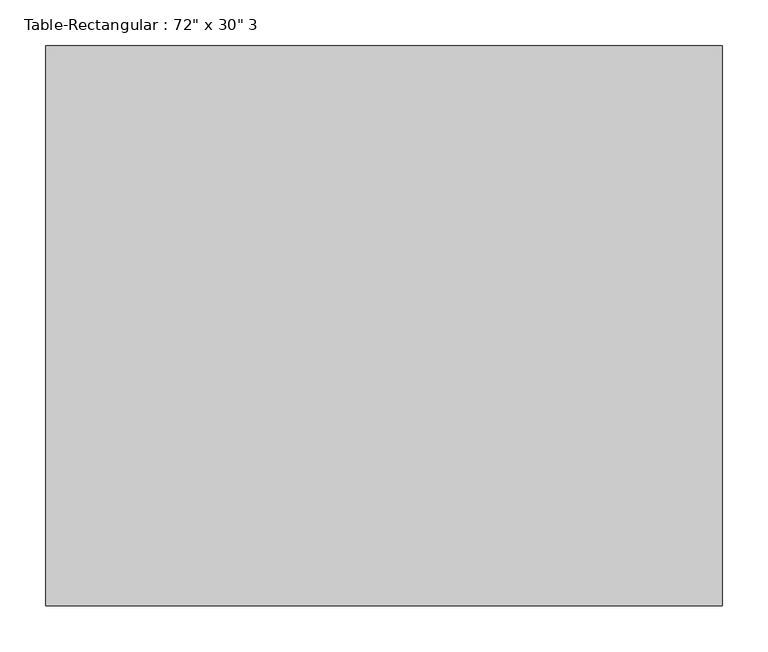
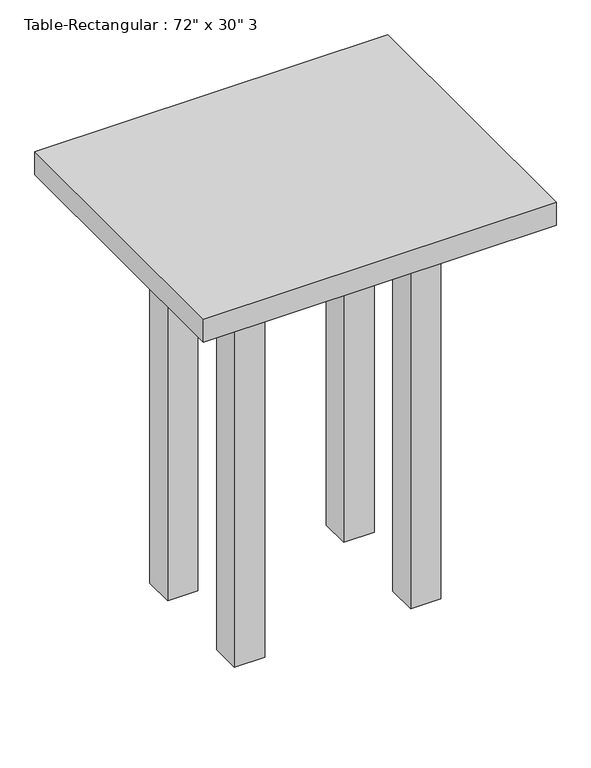
"""IFC4 building model written with IfcOpenShell, lengths in millimetres: furniture geometry."""

from ifc_helpers import new_model, si_unit, frame, origin, origin_with_axes, place, context, project, spatial, polyline, outline, extrude, source, transform, mapped, element, save


def furniture_6a32cbcf(model_context):
    return source(origin(), model_context, "Body", "SweptSolid", [
        extrude(outline(polyline([(152.4, 114.3), (152.4, 88.9), (-152.4, 88.9), (-152.4, 114.3), (152.4, 114.3)])), frame((0.0, 0.0, 762.0), z_axis=(0.0, 0.0, 1.0), x_axis=(1.0, 0.0, 0.0)), (0.0, 0.0, 1.0), 101.6),
        extrude(outline(polyline([(152.4, -114.3), (-152.4, -114.3), (-152.4, -88.9), (152.4, -88.9), (152.4, -114.3)])), frame((0.0, 0.0, 762.0), z_axis=(0.0, 0.0, 1.0), x_axis=(1.0, 0.0, 0.0)), (0.0, 0.0, 1.0), 101.6),
        extrude(outline(polyline([(-165.1, -88.9), (-190.5, -88.9), (-190.5, 88.9), (-165.1, 88.9), (-165.1, -88.9)])), frame((0.0, 0.0, 762.0), z_axis=(0.0, 0.0, 1.0), x_axis=(1.0, 0.0, 0.0)), (0.0, 0.0, 1.0), 101.6),
        extrude(outline(polyline([(165.1, -88.9), (165.1, 88.9), (190.5, 88.9), (190.5, -88.9), (165.1, -88.9)])), frame((0.0, 0.0, 762.0), z_axis=(0.0, 0.0, 1.0), x_axis=(1.0, 0.0, 0.0)), (0.0, 0.0, 1.0), 101.6),
        extrude(outline(polyline([(368.3, 304.8), (368.3, -304.8), (-368.3, -304.8), (-368.3, 304.8), (368.3, 304.8)])), frame((0.0, 0.0, 863.6), z_axis=(0.0, 0.0, 1.0), x_axis=(1.0, 0.0, 0.0)), (0.0, 0.0, 1.0), 50.8),
        extrude(outline(polyline([(-152.4, 152.4), (-152.4, 88.9), (-215.9, 88.9), (-215.9, 152.4), (-152.4, 152.4)])), origin_with_axes(), (0.0, 0.0, 1.0), 863.6),
        extrude(outline(polyline([(152.4, 152.4), (215.9, 152.4), (215.9, 88.9), (152.4, 88.9), (152.4, 152.4)])), origin_with_axes(), (0.0, 0.0, 1.0), 863.6),
        extrude(outline(polyline([(-152.4, -152.4), (-215.9, -152.4), (-215.9, -88.9), (-152.4, -88.9), (-152.4, -152.4)])), origin_with_axes(), (0.0, 0.0, 1.0), 863.6),
        extrude(outline(polyline([(152.4, -152.4), (152.4, -88.9), (215.9, -88.9), (215.9, -152.4), (152.4, -152.4)])), origin_with_axes(), (0.0, 0.0, 1.0), 863.6),
    ])


if __name__ == "__main__":
    model = new_model("IFC4")
    model_context = context("Model", 3, world=origin())
    ifc_project = project(units=[si_unit("LENGTHUNIT", "METRE", prefix="MILLI")], contexts=[model_context])
    site = spatial("IfcSite", under=ifc_project)
    building = spatial("IfcBuilding", under=site)
    placement = place(None, origin())
    furniture_shape = furniture_6a32cbcf(model_context)
    element("IfcFurniture", 1, ObjectType="Table-Rectangular : 72\" x 30\" 3", at=placement, inside=building, context=model_context, shape_type="MappedRepresentation", body=[
        mapped(furniture_shape, transform((0.0, 0.0, 0.0), x_axis=(1.0, 0.0, 0.0), y_axis=(0.0, 1.0, 0.0), z_axis=(0.0, 0.0, 1.0))),
    ])
    save(model, "model.ifc")

# Revit data of these elements
# Type "Table-Rectangular : 72\" x 30\" 3"
#   Assembly Code = "E2020200"
#   Height = 3' - 0"
#   Length = 2' - 5"
#   Width = 2' - 0"
#   Base Material = Birch
#   Top Material = Cherry
#   Default Elevation = 0
# Element 1 (IfcFurniture, "Table-Rectangular : 72\" x 30\" 3")
#   Materials on its faces: "Birch", "Cherry"
# Materials
#   "Birch": class "Wood", colour RGB 224 178 126, transparency 0, Description = "Betula Alleghaniensis", Cost = 0
#   "Cherry": class "Wood", colour RGB 226 177 128, transparency 0, Description = "Prunus Serotina", Cost = 0
